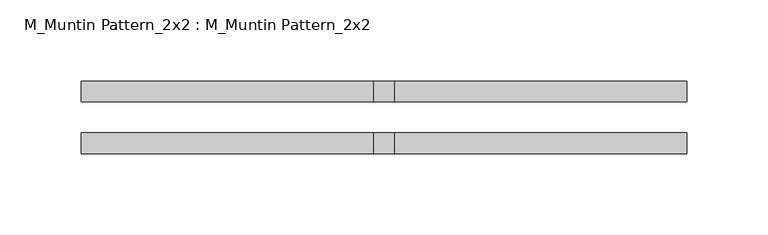
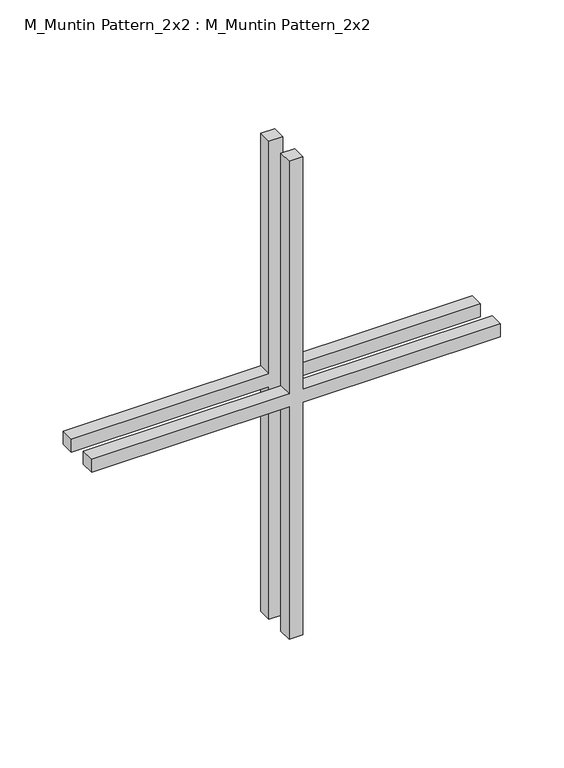
"""IFC4 building model written with IfcOpenShell, lengths in millimetres: proxy geometry, M_Muntin Pattern_2x2 : M_Muntin Pattern_2x2."""

from ifc_helpers import new_model, si_unit, frame, origin, place, context, project, spatial, polyline, outline, extrude, source, transform, mapped, element, save


def m_muntin_pattern_2x2_m_muntin_pattern_2x2_d2526705(model_context):
    return source(origin(), model_context, "Body", "SweptSolid", [
        extrude(outline(polyline([(236.5, -6.35), (236.5, -186.2666667), (223.8, -186.2666667), (223.8, -6.35), (0.0, -6.35), (0.0, 6.35), (223.8, 6.35), (223.8, 186.2666667), (236.5, 186.2666667), (236.5, 6.35), (460.3, 6.35), (460.3, -6.35), (236.5, -6.35)])), frame((0.0, -22.225, 0.0), z_axis=(0.0, 1.0, 0.0), x_axis=(0.0, 0.0, 1.0)), (0.0, 0.0, 1.0), 12.7),
        extrude(outline(polyline([(236.5, -6.35), (236.5, -186.2666667), (223.8, -186.2666667), (223.8, -6.35), (0.0, -6.35), (0.0, 6.35), (223.8, 6.35), (223.8, 186.2666667), (236.5, 186.2666667), (236.5, 6.35), (460.3, 6.35), (460.3, -6.35), (236.5, -6.35)])), frame((0.0, 9.525, 0.0), z_axis=(0.0, 1.0, 0.0), x_axis=(0.0, 0.0, 1.0)), (0.0, 0.0, 1.0), 12.7),
    ])


if __name__ == "__main__":
    model = new_model("IFC4")
    model_context = context("Model", 3, world=origin())
    ifc_project = project(units=[si_unit("LENGTHUNIT", "METRE", prefix="MILLI")], contexts=[model_context])
    site = spatial("IfcSite", under=ifc_project)
    building = spatial("IfcBuilding", under=site)
    placement = place(None, origin())
    m_muntin_pattern_2x2_m_muntin_pattern_2x2_shape = m_muntin_pattern_2x2_m_muntin_pattern_2x2_d2526705(model_context)
    element("IfcBuildingElementProxy", 1, Name="M_Muntin Pattern_2x2 : M_Muntin Pattern_2x2", ObjectType="M_Muntin Pattern_2x2 : M_Muntin Pattern_2x2", at=placement, inside=building, context=model_context, shape_type="MappedRepresentation", body=[
        mapped(m_muntin_pattern_2x2_m_muntin_pattern_2x2_shape, transform((0.0, 0.0, 0.0), x_axis=(1.0, 0.0, 0.0), y_axis=(0.0, 1.0, 0.0), z_axis=(0.0, 0.0, 1.0))),
    ])
    save(model, "model.ifc")

# Revit data of these elements
# Type "M_Muntin Pattern_2x2 : M_Muntin Pattern_2x2"
#   Width [instance default] = 3' - 11.24409"
#   Thickness = 0' - 0 1/2"
#   Height [instance default] = 3' - 11.24409"
#   Distance = 0' - 0 3/4"
#   Interior Material [instance default] = none
#   Exterior Material [instance default] = none
#   Default Elevation = 0
# Element 1 (IfcBuildingElementProxy, "M_Muntin Pattern_2x2 : M_Muntin Pattern_2x2")
#   Width = 1' - 2.66667"
#   Height = 1' - 6.12205"
#   Interior Material = Wood - Stained
#   Exterior Material = Clad - White
#   Materials on its faces: "Clad - White", "Wood - Stained"
# Materials
#   "Clad - White": class "Wood", colour RGB 242 242 238, transparency 0, Cost = 0
#   "Wood - Stained": class "Wood", colour RGB 224 178 126, transparency 0, Cost = 0
